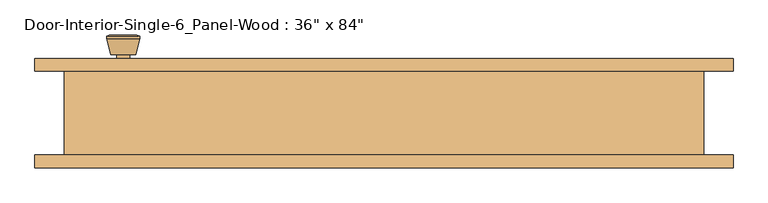
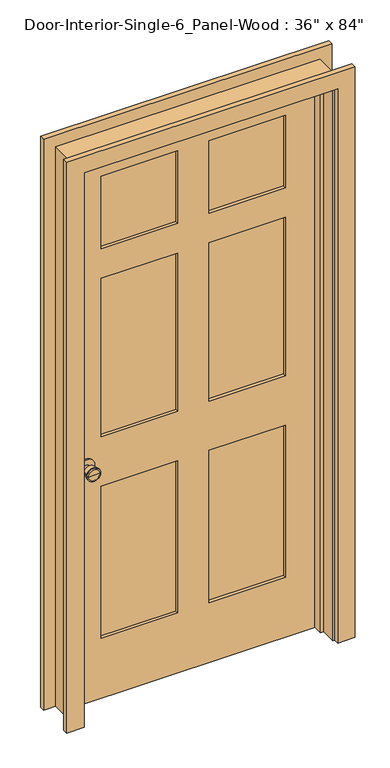
"""IFC4 building model written with IfcOpenShell, lengths in millimetres: door geometry."""

from ifc_helpers import new_model, si_unit, point, frame, frame_2d, origin, place, context, project, spatial, polyline, circle_curve, trimmed, segment, composite_curve, outline, extrude, faceted_brep, source, transform, mapped, element, save
from ifc_brep_helpers import plane_surface, cylinder_surface, revolved_surface, advanced_brep


def door_03e3dfb5(model_context):
    return source(origin(), model_context, "Body", "SolidModel", [
        advanced_brep(
        [(-393.7, 19.4, 914.4), (-383.7, 19.4, 914.4), (-403.7, 19.4, 914.4), (-373.2241324, -29.6, 914.4), (-393.7, -29.6, 914.4), (-414.1758676, -29.6, 914.4), (-368.7, -27.7721319, 914.4), (-418.7, -27.7721319, 914.4), (-368.7, -24.3084537, 914.4), (-418.7, -24.3084537, 914.4), (-375.063764, 0.4, 914.4), (-412.336236, 0.4, 914.4), (-383.7, 0.4, 914.4), (-403.7, 0.4, 914.4)],
        [
            (0, 1),
            (1, 2, circle_curve(frame((-393.7, 19.4, 914.4), z_axis=(0.0, 1.0, 0.0), x_axis=(-1.0, 0.0, 0.0)), 10.0)),
            (2, 0),
            (2, 1, circle_curve(frame((-393.7, 19.4, 914.4), z_axis=(0.0, 1.0, 0.0), x_axis=(-1.0, 0.0, 0.0)), 10.0)),
            (3, 4),
            (4, 5),
            (5, 3, circle_curve(frame((-393.7, -29.6, 914.4), z_axis=(0.0, -1.0, 0.0), x_axis=(-1.0, 0.0, 0.0)), 20.4758676)),
            (3, 5, circle_curve(frame((-393.7, -29.6, 914.4), z_axis=(0.0, -1.0, 0.0), x_axis=(-1.0, 0.0, 0.0)), 20.4758676)),
            (6, 3),
            (5, 7),
            (7, 6, circle_curve(frame((-393.7, -27.7721319, 914.4), z_axis=(0.0, -1.0, 0.0), x_axis=(-1.0, 0.0, 0.0)), 25.0)),
            (6, 7, circle_curve(frame((-393.7, -27.7721319, 914.4), z_axis=(0.0, -1.0, 0.0), x_axis=(-1.0, 0.0, 0.0)), 25.0)),
            (8, 6),
            (7, 9),
            (9, 8, circle_curve(frame((-393.7, -24.3084537, 914.4), z_axis=(0.0, -1.0, 0.0), x_axis=(-1.0, 0.0, 0.0)), 25.0)),
            (8, 9, circle_curve(frame((-393.7, -24.3084537, 914.4), z_axis=(0.0, -1.0, 0.0), x_axis=(-1.0, 0.0, 0.0)), 25.0)),
            (10, 8),
            (9, 11),
            (11, 10, circle_curve(frame((-393.7, 0.4, 914.4), z_axis=(0.0, -1.0, 0.0), x_axis=(-1.0, 0.0, 0.0)), 18.636236)),
            (10, 11, circle_curve(frame((-393.7, 0.4, 914.4), z_axis=(0.0, -1.0, 0.0), x_axis=(-1.0, 0.0, 0.0)), 18.636236)),
            (12, 10),
            (11, 13),
            (13, 12, circle_curve(frame((-393.7, 0.4, 914.4), z_axis=(0.0, -1.0, 0.0), x_axis=(-1.0, 0.0, 0.0)), 10.0)),
            (12, 13, circle_curve(frame((-393.7, 0.4, 914.4), z_axis=(0.0, -1.0, 0.0), x_axis=(-1.0, 0.0, 0.0)), 10.0)),
            (1, 12),
            (13, 2),
        ],
        [
            plane_surface(frame((-393.7, 19.4, 914.4), z_axis=(0.0, 1.0, 0.0), x_axis=(-1.0, 0.0, 0.0))),
            plane_surface(frame((-393.7, -29.6, 914.4), z_axis=(0.0, -1.0, 0.0), x_axis=(-1.0, 0.0, 0.0))),
            revolved_surface(polyline([(-414.1758676, -29.6, 914.4), (-418.7, -27.7721319, 914.4)]), (-393.7, 19.4, 914.4), (0.0, 1.0, 0.0)),
            cylinder_surface(frame((-393.7, 19.4, 914.4), z_axis=(0.0, 1.0, 0.0), x_axis=(-1.0, 0.0, 0.0)), 25.0),
            revolved_surface(polyline([(-418.7, -24.3084537, 914.4), (-412.336236, 0.4, 914.4)]), (-393.7, 19.4, 914.4), (0.0, 1.0, 0.0)),
            plane_surface(frame((-393.7, 0.4, 914.4), z_axis=(0.0, 1.0, 0.0), x_axis=(-1.0, 0.0, 0.0))),
            cylinder_surface(frame((-393.7, 19.4, 914.4), z_axis=(0.0, 1.0, 0.0), x_axis=(-1.0, 0.0, 0.0)), 10.0),
        ],
        [
            (0, [[1, 2, 3]]),
            (0, [[-3, 4, -1]]),
            (1, [[5, 6, 7]]),
            (1, [[-6, -5, 8]]),
            (2, [[9, -7, 10, 11]]),
            (2, [[-10, -8, -9, 12]]),
            (3, [[13, -11, 14, 15]]),
            (3, [[-14, -12, -13, 16]]),
            (4, [[17, -15, 18, 19]]),
            (4, [[-18, -16, -17, 20]]),
            (5, [[21, -19, 22, 23]]),
            (5, [[-22, -20, -21, 24]]),
            (6, [[25, -23, 26, -2]]),
            (6, [[-26, -24, -25, -4]]),
        ],
    ),
        extrude(outline(composite_curve([segment(trimmed(circle_curve(frame_2d((914.4, -393.7)), 30.0), [point((914.4, -423.7))], [point((914.4, -363.7))], False, "CARTESIAN"), True, "CONTINUOUS"), segment(trimmed(circle_curve(frame_2d((914.4, -393.7)), 30.0), [point((914.4, -363.7))], [point((914.4, -423.7))], False, "CARTESIAN"), True, "CONTINUOUS")], self_intersect=False)), frame((0.0, 19.4, 0.0), z_axis=(0.0, 1.0, 0.0), x_axis=(0.0, 0.0, 1.0)), (0.0, 0.0, 1.0), 6.0),
        advanced_brep(
        [(-393.7, 66.325, 914.4), (-403.7, 66.325, 914.4), (-383.7, 66.325, 914.4), (-373.2241324, 115.325, 914.4), (-414.1758676, 115.325, 914.4), (-393.7, 115.325, 914.4), (-368.7, 113.4971319, 914.4), (-418.7, 113.4971319, 914.4), (-368.7, 110.0334537, 914.4), (-418.7, 110.0334537, 914.4), (-375.063764, 85.325, 914.4), (-412.336236, 85.325, 914.4), (-383.7, 85.325, 914.4), (-403.7, 85.325, 914.4)],
        [
            (0, 1),
            (1, 2, circle_curve(frame((-393.7, 66.325, 914.4), z_axis=(0.0, -1.0, 0.0), x_axis=(-1.0, 0.0, 0.0)), 10.0)),
            (2, 0),
            (2, 1, circle_curve(frame((-393.7, 66.325, 914.4), z_axis=(0.0, -1.0, 0.0), x_axis=(-1.0, 0.0, 0.0)), 10.0)),
            (3, 4, circle_curve(frame((-393.7, 115.325, 914.4), z_axis=(0.0, 1.0, 0.0), x_axis=(-1.0, 0.0, 0.0)), 20.4758676)),
            (4, 5),
            (5, 3),
            (4, 3, circle_curve(frame((-393.7, 115.325, 914.4), z_axis=(0.0, 1.0, 0.0), x_axis=(-1.0, 0.0, 0.0)), 20.4758676)),
            (6, 7, circle_curve(frame((-393.7, 113.4971319, 914.4), z_axis=(0.0, 1.0, 0.0), x_axis=(-1.0, 0.0, 0.0)), 25.0)),
            (7, 4),
            (3, 6),
            (7, 6, circle_curve(frame((-393.7, 113.4971319, 914.4), z_axis=(0.0, 1.0, 0.0), x_axis=(-1.0, 0.0, 0.0)), 25.0)),
            (8, 9, circle_curve(frame((-393.7, 110.0334537, 914.4), z_axis=(0.0, 1.0, 0.0), x_axis=(-1.0, 0.0, 0.0)), 25.0)),
            (9, 7),
            (6, 8),
            (9, 8, circle_curve(frame((-393.7, 110.0334537, 914.4), z_axis=(0.0, 1.0, 0.0), x_axis=(-1.0, 0.0, 0.0)), 25.0)),
            (10, 11, circle_curve(frame((-393.7, 85.325, 914.4), z_axis=(0.0, 1.0, 0.0), x_axis=(-1.0, 0.0, 0.0)), 18.636236)),
            (11, 9),
            (8, 10),
            (11, 10, circle_curve(frame((-393.7, 85.325, 914.4), z_axis=(0.0, 1.0, 0.0), x_axis=(-1.0, 0.0, 0.0)), 18.636236)),
            (12, 13, circle_curve(frame((-393.7, 85.325, 914.4), z_axis=(0.0, 1.0, 0.0), x_axis=(-1.0, 0.0, 0.0)), 10.0)),
            (13, 11),
            (10, 12),
            (13, 12, circle_curve(frame((-393.7, 85.325, 914.4), z_axis=(0.0, 1.0, 0.0), x_axis=(-1.0, 0.0, 0.0)), 10.0)),
            (1, 13),
            (12, 2),
        ],
        [
            plane_surface(frame((-393.7, 66.325, 914.4), z_axis=(0.0, -1.0, 0.0), x_axis=(-1.0, 0.0, 0.0))),
            plane_surface(frame((-393.7, 115.325, 914.4), z_axis=(0.0, 1.0, 0.0), x_axis=(-1.0, 0.0, 0.0))),
            revolved_surface(polyline([(-414.1758676, 115.325, 914.4), (-418.7, 113.4971319, 914.4)]), (-393.7, 66.325, 914.4), (0.0, -1.0, 0.0)),
            cylinder_surface(frame((-393.7, 66.325, 914.4), z_axis=(0.0, -1.0, 0.0), x_axis=(-1.0, 0.0, 0.0)), 25.0),
            revolved_surface(polyline([(-418.7, 110.0334537, 914.4), (-412.336236, 85.325, 914.4)]), (-393.7, 66.325, 914.4), (0.0, -1.0, 0.0)),
            plane_surface(frame((-393.7, 85.325, 914.4), z_axis=(0.0, -1.0, 0.0), x_axis=(-1.0, 0.0, 0.0))),
            cylinder_surface(frame((-393.7, 66.325, 914.4), z_axis=(0.0, -1.0, 0.0), x_axis=(-1.0, 0.0, 0.0)), 10.0),
        ],
        [
            (0, [[1, 2, 3]]),
            (0, [[-3, 4, -1]]),
            (1, [[5, 6, 7]]),
            (1, [[8, -7, -6]]),
            (2, [[9, 10, -5, 11]]),
            (2, [[12, -11, -8, -10]]),
            (3, [[13, 14, -9, 15]]),
            (3, [[16, -15, -12, -14]]),
            (4, [[17, 18, -13, 19]]),
            (4, [[20, -19, -16, -18]]),
            (5, [[21, 22, -17, 23]]),
            (5, [[24, -23, -20, -22]]),
            (6, [[-2, 25, -21, 26]]),
            (6, [[-4, -26, -24, -25]]),
        ],
    ),
        extrude(outline(composite_curve([segment(trimmed(circle_curve(frame_2d((914.4, -393.7)), 30.0), [point((914.4, -423.7))], [point((914.4, -363.7))], False, "CARTESIAN"), True, "CONTINUOUS"), segment(trimmed(circle_curve(frame_2d((914.4, -393.7)), 30.0), [point((914.4, -363.7))], [point((914.4, -423.7))], False, "CARTESIAN"), True, "CONTINUOUS")], self_intersect=False)), frame((0.0, 60.325, 0.0), z_axis=(0.0, 1.0, 0.0), x_axis=(0.0, 0.0, 1.0)), (0.0, 0.0, 1.0), 6.0),
        faceted_brep([(482.6, 60.325, 0.0), (482.6, -66.675, 0.0), (457.2, -66.675, 0.0), (457.2, -9.525, 0.0), (444.5, -9.525, 0.0), (444.5, 25.4, 0.0), (457.2, 25.4, 0.0), (457.2, 60.325, 0.0), (482.6, 60.325, 2159.0), (482.6, -66.675, 2159.0), (-482.6, -66.675, 2159.0), (-482.6, -66.675, 0.0), (-457.2, -66.675, 0.0), (-457.2, -66.675, 2133.6), (457.2, -66.675, 2133.6), (457.2, -9.525, 2133.6), (-457.2, -9.525, 2133.6), (-457.2, -9.525, 0.0), (-444.5, -9.525, 0.0), (-444.5, -9.525, 2120.9), (444.5, -9.525, 2120.9), (444.5, 25.4, 2120.9), (-444.5, 25.4, 2120.9), (-444.5, 25.4, 0.0), (-457.2, 25.4, 0.0), (-457.2, 25.4, 2133.6), (457.2, 25.4, 2133.6), (457.2, 60.325, 2133.6), (-457.2, 60.325, 2133.6), (-457.2, 60.325, 0.0), (-482.6, 60.325, 0.0), (-482.6, 60.325, 2159.0)], [[[0, 1, 2, 3, 4, 5, 6, 7]], [[1, 0, 8, 9]], [[2, 1, 9, 10, 11, 12, 13, 14]], [[3, 2, 14, 15]], [[4, 3, 15, 16, 17, 18, 19, 20]], [[5, 4, 20, 21]], [[6, 5, 21, 22, 23, 24, 25, 26]], [[7, 6, 26, 27]], [[0, 7, 27, 28, 29, 30, 31, 8]], [[9, 8, 31, 10]], [[15, 14, 13, 16]], [[21, 20, 19, 22]], [[27, 26, 25, 28]], [[30, 29, 24, 23, 18, 17, 12, 11]], [[10, 31, 30, 11]], [[16, 13, 12, 17]], [[22, 19, 18, 23]], [[28, 25, 24, 29]]]),
        extrude(outline(polyline([(2133.6, -457.2), (0.0, -457.2), (0.0, 457.2), (2133.6, 457.2), (2133.6, -457.2)]), holes=[polyline([(2014.5375, 57.15), (2014.5375, 336.55), (1735.1375, 336.55), (1735.1375, 57.15), (2014.5375, 57.15)]), polyline([(1620.8375, 336.55), (1009.65, 336.55), (1009.65, 57.15), (1620.8375, 57.15), (1620.8375, 336.55)]), polyline([(1009.65, -57.15), (1009.65, -336.55), (1620.8375, -336.55), (1620.8375, -57.15), (1009.65, -57.15)]), polyline([(1735.1375, -336.55), (2014.5375, -336.55), (2014.5375, -57.15), (1735.1375, -57.15), (1735.1375, -336.55)]), polyline([(819.15, 57.15), (819.15, 336.55), (231.775, 336.55), (231.775, 57.15), (819.15, 57.15)]), polyline([(231.775, -57.15), (231.775, -336.55), (819.15, -336.55), (819.15, -57.15), (231.775, -57.15)])]), frame((0.0, 25.4, 0.0), z_axis=(0.0, 1.0, 0.0), x_axis=(0.0, 0.0, 1.0)), (0.0, 0.0, 1.0), 34.925),
        extrude(outline(polyline([(336.55, 37.0416667), (57.15, 37.0416667), (57.15, 48.6833333), (336.55, 48.6833333), (336.55, 37.0416667)])), frame((0.0, 0.0, 1735.1375), z_axis=(0.0, 0.0, 1.0), x_axis=(1.0, 0.0, 0.0)), (0.0, 0.0, 1.0), 279.4),
        extrude(outline(polyline([(336.55, 37.0416667), (57.15, 37.0416667), (57.15, 48.6833333), (336.55, 48.6833333), (336.55, 37.0416667)])), frame((0.0, 0.0, 1009.65), z_axis=(0.0, 0.0, 1.0), x_axis=(1.0, 0.0, 0.0)), (0.0, 0.0, 1.0), 611.1875),
        extrude(outline(polyline([(-57.15, 37.0416667), (-336.55, 37.0416667), (-336.55, 48.6833333), (-57.15, 48.6833333), (-57.15, 37.0416667)])), frame((0.0, 0.0, 1009.65), z_axis=(0.0, 0.0, 1.0), x_axis=(1.0, 0.0, 0.0)), (0.0, 0.0, 1.0), 611.1875),
        extrude(outline(polyline([(-57.15, 37.0416667), (-336.55, 37.0416667), (-336.55, 48.6833333), (-57.15, 48.6833333), (-57.15, 37.0416667)])), frame((0.0, 0.0, 1735.1375), z_axis=(0.0, 0.0, 1.0), x_axis=(1.0, 0.0, 0.0)), (0.0, 0.0, 1.0), 279.4),
        extrude(outline(polyline([(336.55, 37.0416667), (57.15, 37.0416667), (57.15, 48.6833333), (336.55, 48.6833333), (336.55, 37.0416667)])), frame((0.0, 0.0, 231.775), z_axis=(0.0, 0.0, 1.0), x_axis=(1.0, 0.0, 0.0)), (0.0, 0.0, 1.0), 587.375),
        extrude(outline(polyline([(-57.15, 37.0416667), (-336.55, 37.0416667), (-336.55, 48.6833333), (-57.15, 48.6833333), (-57.15, 37.0416667)])), frame((0.0, 0.0, 231.775), z_axis=(0.0, 0.0, 1.0), x_axis=(1.0, 0.0, 0.0)), (0.0, 0.0, 1.0), 587.375),
        extrude(outline(polyline([(0.0, 463.55), (0.0, 527.05), (2203.45, 527.05), (2203.45, -527.05), (0.0, -527.05), (0.0, -463.55), (2139.95, -463.55), (2139.95, 463.55), (0.0, 463.55)])), frame((0.0, 60.325, 0.0), z_axis=(0.0, 1.0, 0.0), x_axis=(0.0, 0.0, 1.0)), (0.0, 0.0, 1.0), 19.05),
        extrude(outline(polyline([(0.0, 463.55), (0.0, 527.05), (2203.45, 527.05), (2203.45, -527.05), (0.0, -527.05), (0.0, -463.55), (2139.95, -463.55), (2139.95, 463.55), (0.0, 463.55)])), frame((0.0, -85.725, 0.0), z_axis=(0.0, 1.0, 0.0), x_axis=(0.0, 0.0, 1.0)), (0.0, 0.0, 1.0), 19.05),
    ])


if __name__ == "__main__":
    model = new_model("IFC4")
    model_context = context("Model", 3, world=origin())
    ifc_project = project(units=[si_unit("LENGTHUNIT", "METRE", prefix="MILLI")], contexts=[model_context])
    site = spatial("IfcSite", under=ifc_project)
    building = spatial("IfcBuilding", under=site)
    placement = place(None, origin())
    door_shape = door_03e3dfb5(model_context)
    element("IfcDoor", 1, ObjectType="Door-Interior-Single-6_Panel-Wood : 36\" x 84\"", at=placement, inside=building, context=model_context, shape_type="MappedRepresentation", body=[
        mapped(door_shape, transform((0.0, 0.0, 0.0), x_axis=(1.0, 0.0, 0.0), y_axis=(0.0, 1.0, 0.0), z_axis=(0.0, 0.0, 1.0))),
    ])
    save(model, "model.ifc")

# Revit data of these elements
# Type "Door-Interior-Single-6_Panel-Wood : 36\" x 84\""
#   Type Mark = "10"
#   Assembly Code = "C1020300"
#   Analytic Construction = "Wooden"
#   Top Rail = 0' - 4 11/16"
#   Top Panel = 0' - 11"
#   Thickness = 0' - 1 3/8"
#   Thermal Resistance (R) = 2.5876 (h·ft²·°F)/BTU
#   Swing Angle [instance default] = 90.00°
#   Stiles = 0' - 4 3/4"
#   Rough Width = 3' - 2"
#   Rough Height = 7' - 1"
#   Mullion = 0' - 4 1/2"
#   Lock Rail = 0' - 7 1/2"
#   Intermediate Rail = 0' - 4 1/2"
#   Height = 7' - 0"
#   Width = 3' - 0"
#   Heat Transfer Coefficient (U) = 0.3865 BTU/(h·ft²·°F)
#   Bottom Rail = 0' - 9 1/8"
#   Trim Material = Cherry
#   Panel Material = Cherry
#   Frame Material = Cherry
#   Door Handle Material = Aluminum
#   Visual Light Transmittance = 0
#   Solar Heat Gain Coefficient = 0
#   Wall Closure = (empty or 0)
#   Function = (empty or 0)
# Element 1 (IfcDoor, "Door-Interior-Single-6_Panel-Wood : 36\" x 84\"")
#   Materials on its faces: "Cherry", "Aluminum"
# Materials
#   "Cherry": class "Wood", colour RGB 226 177 128, transparency 0, Description = "Prunus Serotina", Cost = 0
#   "Aluminum": class "Metal", colour RGB 247 247 247, transparency 0, Description = "Aluminum 6061", Cost = 0
